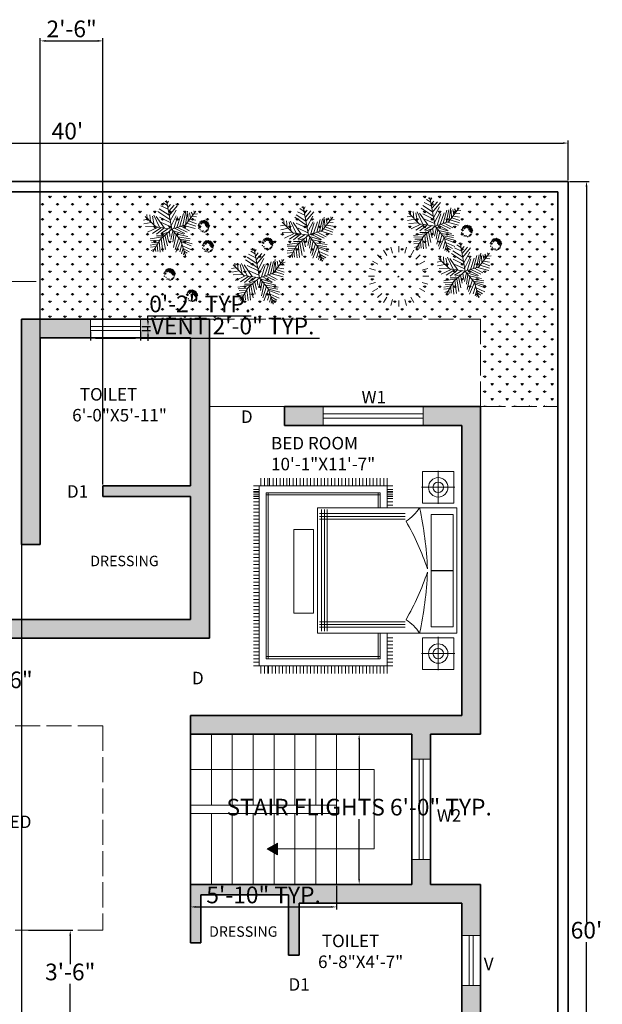
# Model space of a CAD drawing. Units: inches. Extents: x 1070 to 2371, y 645 to 1546.
# Tile 7 of 10: x 1379 to 1658, y 1014 to 1486. Entities that reach past the tile are written whole.
import ezdxf

# ---------------------------------------------------------------- set-up
doc = ezdxf.new("R2010")
doc.units = ezdxf.units.IN
doc.linetypes.add('ACAD_ISO02W100', pattern=[15, 12, -3])
for name, color, linetype, lineweight in [('A-ANNO-DIMS', 2, 'Continuous', 18), ('A-ANNO-SYMB', 7, 'Continuous', 18), ('A-ANNO-TEXT', 7, 'Continuous', 18), ('A-AREA-IDEN', 7, 'Continuous', 18), ('A-DOOR', 4, 'Continuous', 18), ('A-FLOR-OVHD', 8, 'ACAD_ISO02W100', 13), ('A-FLOR-STRS', 7, 'Continuous', 18), ('A-FURN', 8, 'Continuous', 18), ('A-GLAZ', 4, 'Continuous', 18), ('A-ROOF-OVHD', 8, 'ACAD_ISO02W100', 13), ('A-WALL', 7, 'Continuous', 35), ('C-PROP', 7, 'Continuous', 35), ('L-PLNT-BEDS-HIDN', 3, 'ACAD_ISO02W100', 13), ('L-PLNT-TREE', 94, 'Continuous', 13)]:
    doc.layers.add(name, color=color, linetype=linetype, lineweight=lineweight)
doc.layers.add('A-WALL-PATT', color=162, linetype='Continuous', lineweight=13, true_color=0x044ac3)
doc.layers.add('L-PLNT-PATT', color=85, linetype='Continuous', lineweight=13, true_color=0x58ba48)
doc.styles.get("Standard").update_dxf_attribs({"font": 'arial.ttf'})
doc.dimstyles.new('ISO-25', dxfattribs={"dimtxt": 8, "dimasz": 2.5, "dimexe": 1.25, "dimexo": 0.625, "dimtad": 1, "dimtih": 1, "dimtoh": 1, "dimdec": 1, "dimlunit": 3, "dimtxsty": 'Standard', "dimcen": 2.5, "dimadec": 0, "dimazin": 0, "dimtfac": 1, "dimtdec": 1, "dimtmove": 0, "dimatfit": 3, "dimfxl": 1, "dimarcsym": 0})

# ---------------------------------------------------------------- blocks, each defined once
blk = doc.blocks.new('A$C462B680F')
for p, q in [((0.011, 2.874, -0.291), (0.465, 2.874, -0.291)), ((0.011, 2.424, -0.291), (0.011, 2.874, -0.291)), ((0.238, 2.649, -0.561), (0.238, 2.887, -0.561)), ((0.465, 2.874, -0.291), (0.465, 2.424, -0.291)), ((2.33, 2.918, -0.291), (0.53, 2.918, -0.291)), ((0.53, 2.918, -0.291), (0.53, 0.918, -0.291)), ((1.434, 2.861, -0.291), (0.627, 2.861, -0.291)), ((0.627, 2.861, -0.291), (0.627, 2.55, -0.291)), ((1.43, 2.861, -0.291), (1.43, 2.55, -0.291)), ((2.237, 2.861, -0.291), (1.43, 2.861, -0.291)), ((1.434, 2.55, -0.291), (1.434, 2.861, -0.291)), ((2.237, 2.55, -0.291), (2.237, 2.861, -0.291)), ((2.33, 0.918, -0.291), (2.33, 2.918, -0.291)), ((2.849, 2.874, -0.291), (2.395, 2.874, -0.291)), ((2.395, 2.874, -0.291), (2.395, 2.424, -0.291)), ((2.622, 2.649, -0.561), (2.622, 2.887, -0.561)), ((2.849, 2.424, -0.291), (2.849, 2.874, -0.291)), ((0.238, 2.649, -0.561), (0, 2.649, -0.561)), ((0.238, 2.649, -0.561), (0.238, 2.411, -0.561)), ((0.238, 2.649, -0.561), (0.476, 2.649, -0.561)), ((0.627, 2.55, -0.291), (1.434, 2.55, -0.291)), ((1.43, 2.55, -0.291), (2.237, 2.55, -0.291)), ((2.622, 2.649, -0.561), (2.384, 2.649, -0.561)), ((2.622, 2.649, -0.561), (2.622, 2.411, -0.561)), ((2.622, 2.649, -0.561), (2.861, 2.649, -0.561)), ((0.465, 2.424, -0.291), (0.011, 2.424, -0.291)), ((2.395, 2.424, -0.291), (2.849, 2.424, -0.291)), ((0.615, 2.176, -0.291), (0.615, 0.947, -0.291)), ((0.655, 2.176, -0.291), (0.655, 0.947, -0.291)), ((0.695, 2.176, -0.291), (0.695, 0.947, -0.291)), ((2.165, 2.176, -0.291), (2.165, 0.947, -0.291)), ((2.205, 2.176, -0.291), (2.205, 0.947, -0.291)), ((2.245, 2.176, -0.291), (2.245, 0.947, -0.291)), ((0.219, 1.918, -0.291), (0.219, 2, -0.291)), ((0.269, 1.918, -0.291), (0.269, 2, -0.291)), ((0.296, 1.918, -0.291), (0.296, 2, -0.291)), ((0.319, 1.918, -0.291), (0.319, 2, -0.291)), ((0.346, 1.918, -0.291), (0.346, 2, -0.291)), ((0.369, 1.918, -0.291), (0.369, 2, -0.291)), ((0.396, 1.918, -0.291), (0.396, 2, -0.291)), ((0.446, 1.918, -0.291), (0.446, 2, -0.291)), ((0.496, 1.918, -0.291), (0.496, 2, -0.291)), ((2.396, 1.918, -0.291), (2.396, 2, -0.291)), ((2.446, 1.918, -0.291), (2.446, 2, -0.291)), ((2.496, 1.918, -0.291), (2.496, 2, -0.291)), ((2.546, 1.918, -0.291), (2.546, 2, -0.291)), ((2.596, 1.918, -0.291), (2.596, 2, -0.291)), ((2.646, 1.918, -0.291), (2.646, 2, -0.291)), ((2.696, 1.918, -0.291), (2.696, 2, -0.291)), ((2.746, 1.918, -0.291), (2.746, 2, -0.291)), ((2.796, 1.918, -0.291), (2.796, 2, -0.291)), ((0.215, 1.918, -0.291), (0.105, 1.918, -0.291)), ((0.215, 1.868, -0.291), (0.105, 1.868, -0.291)), ((0.215, 1.918, -0.291), (0.215, 0.082, -0.291)), ((0.53, 1.918, -0.291), (0.215, 1.918, -0.291)), ((2.33, 1.918, -0.291), (2.796, 1.918, -0.291)), ((2.796, 1.918, -0.291), (2.796, 0.082, -0.291)), ((2.796, 1.918, -0.291), (2.906, 1.918, -0.291)), ((2.796, 1.868, -0.291), (2.906, 1.868, -0.291)), ((0.215, 1.818, -0.291), (0.105, 1.818, -0.291)), ((0.215, 1.768, -0.291), (0.105, 1.768, -0.291)), ((0.215, 1.718, -0.291), (0.105, 1.718, -0.291)), ((0.315, 1.818, -0.291), (0.315, 0.182, -0.291)), ((0.53, 1.818, -0.291), (0.315, 1.818, -0.291)), ((0.53, 1.788, -0.291), (0.315, 1.788, -0.291)), ((0.345, 1.818, -0.291), (0.345, 0.182, -0.291)), ((2.33, 1.818, -0.291), (2.696, 1.818, -0.291)), ((2.33, 1.788, -0.291), (2.696, 1.788, -0.291)), ((2.666, 1.818, -0.291), (2.666, 0.182, -0.291)), ((2.696, 1.818, -0.291), (2.696, 0.182, -0.291)), ((2.796, 1.818, -0.291), (2.906, 1.818, -0.291)), ((2.796, 1.768, -0.291), (2.906, 1.768, -0.291)), ((2.796, 1.718, -0.291), (2.906, 1.718, -0.291)), ((0.215, 1.668, -0.291), (0.105, 1.668, -0.291)), ((0.215, 1.618, -0.291), (0.105, 1.618, -0.291)), ((0.215, 1.568, -0.291), (0.105, 1.568, -0.291)), ((2.796, 1.668, -0.291), (2.906, 1.668, -0.291)), ((2.796, 1.618, -0.291), (2.906, 1.618, -0.291)), ((2.796, 1.568, -0.291), (2.906, 1.568, -0.291)), ((0.215, 1.518, -0.291), (0.105, 1.518, -0.291)), ((0.215, 1.468, -0.291), (0.105, 1.468, -0.291)), ((0.215, 1.418, -0.291), (0.105, 1.418, -0.291)), ((2.796, 1.518, -0.291), (2.906, 1.518, -0.291)), ((2.796, 1.468, -0.291), (2.906, 1.468, -0.291)), ((2.796, 1.418, -0.291), (2.906, 1.418, -0.291)), ((0.215, 1.368, -0.291), (0.105, 1.368, -0.291)), ((0.215, 1.318, -0.291), (0.105, 1.318, -0.291)), ((2.796, 1.368, -0.291), (2.906, 1.368, -0.291)), ((2.796, 1.318, -0.291), (2.906, 1.318, -0.291)), ((0.215, 1.268, -0.291), (0.105, 1.268, -0.291)), ((0.215, 1.218, -0.291), (0.105, 1.218, -0.291)), ((0.215, 1.168, -0.291), (0.105, 1.168, -0.291)), ((2.796, 1.268, -0.291), (2.906, 1.268, -0.291)), ((2.796, 1.218, -0.291), (2.906, 1.218, -0.291)), ((2.796, 1.168, -0.291), (2.906, 1.168, -0.291)), ((0.215, 1.118, -0.291), (0.105, 1.118, -0.291)), ((0.215, 1.068, -0.291), (0.105, 1.068, -0.291)), ((0.215, 1.018, -0.291), (0.105, 1.018, -0.291)), ((0.558, 1.057, -0.291), (2.299, 1.057, -0.291)), ((0.558, 1.017, -0.291), (2.299, 1.017, -0.291)), ((2.796, 1.118, -0.291), (2.906, 1.118, -0.291)), ((2.796, 1.068, -0.291), (2.906, 1.068, -0.291)), ((2.796, 1.018, -0.291), (2.906, 1.018, -0.291)), ((0.215, 0.968, -0.291), (0.105, 0.968, -0.291)), ((0.215, 0.918, -0.291), (0.105, 0.918, -0.291)), ((0.215, 0.868, -0.291), (0.105, 0.868, -0.291)), ((0.53, 0.918, -0.291), (2.33, 0.918, -0.291)), ((0.558, 0.977, -0.291), (2.299, 0.977, -0.291)), ((0.844, 0.859, -0.291), (0.844, 0.579, -0.291)), ((2.044, 0.859, -0.291), (0.844, 0.859, -0.291)), ((2.044, 0.579, -0.291), (2.044, 0.859, -0.291)), ((2.796, 0.968, -0.291), (2.906, 0.968, -0.291)), ((2.796, 0.918, -0.291), (2.906, 0.918, -0.291)), ((2.796, 0.868, -0.291), (2.906, 0.868, -0.291)), ((0.215, 0.818, -0.291), (0.105, 0.818, -0.291)), ((0.215, 0.768, -0.291), (0.105, 0.768, -0.291)), ((0.215, 0.718, -0.291), (0.105, 0.718, -0.291)), ((2.796, 0.818, -0.291), (2.906, 0.818, -0.291)), ((2.796, 0.768, -0.291), (2.906, 0.768, -0.291)), ((2.796, 0.718, -0.291), (2.906, 0.718, -0.291)), ((0.215, 0.668, -0.291), (0.105, 0.668, -0.291)), ((0.215, 0.618, -0.291), (0.105, 0.618, -0.291)), ((0.215, 0.568, -0.291), (0.105, 0.568, -0.291)), ((0.844, 0.579, -0.291), (2.044, 0.579, -0.291)), ((2.796, 0.668, -0.291), (2.906, 0.668, -0.291)), ((2.796, 0.618, -0.291), (2.906, 0.618, -0.291)), ((2.796, 0.568, -0.291), (2.906, 0.568, -0.291)), ((0.215, 0.518, -0.291), (0.105, 0.518, -0.291)), ((0.215, 0.48, -0.291), (0.105, 0.48, -0.291)), ((0.215, 0.43, -0.291), (0.105, 0.43, -0.291)), ((2.796, 0.518, -0.291), (2.906, 0.518, -0.291)), ((2.796, 0.516, -0.291), (2.906, 0.516, -0.291)), ((2.796, 0.466, -0.291), (2.906, 0.466, -0.291)), ((0.215, 0.38, -0.291), (0.105, 0.38, -0.291)), ((0.215, 0.33, -0.291), (0.105, 0.33, -0.291)), ((2.796, 0.416, -0.291), (2.906, 0.416, -0.291)), ((2.796, 0.366, -0.291), (2.906, 0.366, -0.291)), ((2.796, 0.316, -0.291), (2.906, 0.316, -0.291)), ((0.215, 0.28, -0.291), (0.105, 0.28, -0.291)), ((0.215, 0.23, -0.291), (0.105, 0.23, -0.291)), ((0.215, 0.207, -0.291), (0.105, 0.207, -0.291)), ((0.215, 0.207, -0.291), (0.105, 0.207, -0.291)), ((0.215, 0.157, -0.291), (0.105, 0.157, -0.291)), ((2.696, 0.212, -0.291), (0.315, 0.212, -0.291)), ((2.696, 0.182, -0.291), (0.315, 0.182, -0.291)), ((2.796, 0.266, -0.291), (2.906, 0.266, -0.291)), ((2.796, 0.216, -0.291), (2.906, 0.216, -0.291)), ((2.796, 0.207, -0.291), (2.906, 0.207, -0.291)), ((2.796, 0.207, -0.291), (2.906, 0.207, -0.291)), ((2.796, 0.157, -0.291), (2.906, 0.157, -0.291)), ((0.215, 0.107, -0.291), (0.105, 0.107, -0.291)), ((2.796, 0.082, -0.291), (0.215, 0.082, -0.291)), ((0.219, 0.082, -0.291), (0.219, 0, -0.291)), ((0.269, 0.082, -0.291), (0.269, 0, -0.291)), ((0.296, 0.082, -0.291), (0.296, 0, -0.291)), ((0.319, 0.082, -0.291), (0.319, 0, -0.291)), ((0.346, 0.082, -0.291), (0.346, 0, -0.291)), ((0.369, 0.082, -0.291), (0.369, 0, -0.291)), ((0.396, 0.082, -0.291), (0.396, 0, -0.291)), ((0.446, 0.082, -0.291), (0.446, 0, -0.291)), ((0.496, 0.082, -0.291), (0.496, 0, -0.291)), ((0.546, 0.082, -0.291), (0.546, 0, -0.291)), ((0.596, 0.082, -0.291), (0.596, 0, -0.291)), ((0.646, 0.082, -0.291), (0.646, 0, -0.291)), ((0.696, 0.082, -0.291), (0.696, 0, -0.291)), ((0.746, 0.082, -0.291), (0.746, 0, -0.291)), ((0.796, 0.082, -0.291), (0.796, 0, -0.291)), ((0.846, 0.082, -0.291), (0.846, 0, -0.291)), ((0.896, 0.082, -0.291), (0.896, 0, -0.291)), ((0.946, 0.082, -0.291), (0.946, 0, -0.291)), ((0.996, 0.082, -0.291), (0.996, 0, -0.291)), ((1.046, 0.082, -0.291), (1.046, 0, -0.291)), ((1.096, 0.082, -0.291), (1.096, 0, -0.291)), ((1.146, 0.082, -0.291), (1.146, 0, -0.291)), ((1.196, 0.082, -0.291), (1.196, 0, -0.291)), ((1.246, 0.082, -0.291), (1.246, 0, -0.291)), ((1.296, 0.082, -0.291), (1.296, 0, -0.291)), ((1.346, 0.082, -0.291), (1.346, 0, -0.291)), ((1.346, 0.082, -0.291), (1.346, 0, -0.291)), ((1.396, 0.082, -0.291), (1.396, 0, -0.291)), ((1.396, 0.082, -0.291), (1.396, 0, -0.291)), ((1.446, 0.082, -0.291), (1.446, 0, -0.291)), ((1.446, 0.082, -0.291), (1.446, 0, -0.291)), ((1.496, 0.082, -0.291), (1.496, 0, -0.291)), ((1.496, 0.082, -0.291), (1.496, 0, -0.291)), ((1.546, 0.082, -0.291), (1.546, 0, -0.291)), ((1.596, 0.082, -0.291), (1.596, 0, -0.291)), ((1.646, 0.082, -0.291), (1.646, 0, -0.291)), ((1.696, 0.082, -0.291), (1.696, 0, -0.291)), ((1.746, 0.082, -0.291), (1.746, 0, -0.291)), ((1.796, 0.082, -0.291), (1.796, 0, -0.291)), ((1.846, 0.082, -0.291), (1.846, 0, -0.291)), ((1.846, 0.082, -0.291), (1.846, 0, -0.291)), ((1.896, 0.082, -0.291), (1.896, 0, -0.291)), ((1.946, 0.082, -0.291), (1.946, 0, -0.291)), ((1.996, 0.082, -0.291), (1.996, 0, -0.291)), ((2.046, 0.082, -0.291), (2.046, 0, -0.291)), ((2.096, 0.082, -0.291), (2.096, 0, -0.291)), ((2.146, 0.082, -0.291), (2.146, 0, -0.291)), ((2.196, 0.082, -0.291), (2.196, 0, -0.291)), ((2.246, 0.082, -0.291), (2.246, 0, -0.291)), ((2.296, 0.082, -0.291), (2.296, 0, -0.291)), ((2.346, 0.082, -0.291), (2.346, 0, -0.291)), ((2.396, 0.082, -0.291), (2.396, 0, -0.291)), ((2.446, 0.082, -0.291), (2.446, 0, -0.291)), ((2.496, 0.082, -0.291), (2.496, 0, -0.291)), ((2.546, 0.082, -0.291), (2.546, 0, -0.291)), ((2.596, 0.082, -0.291), (2.596, 0, -0.291)), ((2.646, 0.082, -0.291), (2.646, 0, -0.291)), ((2.696, 0.082, -0.291), (2.696, 0, -0.291)), ((2.746, 0.082, -0.291), (2.746, 0, -0.291)), ((2.796, 0.107, -0.291), (2.906, 0.107, -0.291)), ((2.796, 0.082, -0.291), (2.796, 0, -0.291))]:
    blk.add_line(p, q)
for centre, radius in [((0.238, 2.649, -0.561), 0.139), ((0.238, 2.649, -0.561), 0.075), ((2.622, 2.649, -0.561), 0.139), ((2.622, 2.649, -0.561), 0.075)]:
    blk.add_circle(centre, radius)
for centre, radius, start, end in [((1.618, -2.572, -0.291), 5.071, 92.3872, 102.3913), ((2.601, -1.074, -0.291), 3.763, 108.5127, 119.9306), ((1.243, -2.572, -0.291), 5.071, 77.6087, 87.6128), ((0.259, -1.074, -0.291), 3.763, 60.0694, 71.4873), ((0.231, 1.886, -0.291), 0.578, 31.4118, 58.8491), ((2.63, 1.886, -0.291), 0.578, 121.1509, 148.5882)]:
    blk.add_arc(centre, radius, start, end)
blk = doc.blocks.new('*U5')
for p, q in [((-5.114, 28.097), (-24.676, 40.636)), ((-7.288, 39.707), (-21.778, 46.673)), ((-8.737, 47.138), (-17.069, 52.711)), ((-10.186, 53.64), (-13.084, 55.962)), ((0, 0), (-10.5, 57)), ((-9.099, 51.782), (-6.563, 55.962)), ((-7.65, 43.423), (-2.578, 49.46)), ((-5.839, 35.992), (4.667, 48.067)), ((-5.114, 27.632), (10.463, 46.673)), ((-47.498, 19.737), (-55.83, 18.344)), ((-31.5, 4.5), (-52.5, 25.5)), ((-48.585, 21.131), (-49.309, 29.026)), ((-43.513, 28.561), (-42.427, 15.558)), ((-38.442, 26.239), (-34.819, 7.663)), ((-35.544, 28.097), (-24.314, 3.947)), ((-14.533, 2.09), (-30.834, 25.31)), ((-3.665, 19.273), (-27.574, 35.527)), ((-24.314, 23.917), (-2.941, 13.7)), ((-2.941, 16.486), (8.652, 37.85)), ((-1.129, 6.734), (9.014, 26.704)), ((3.942, 1.625), (11.187, 24.381)), ((10.101, 3.483), (17.708, 26.239)), ((16.259, 5.805), (23.142, 31.348)), ((22.055, 7.198), (27.489, 32.277)), ((27, 9), (48, 36)), ((27.127, 9.056), (31.112, 35.992)), ((31.836, 30.883), (32.561, 16.486)), ((35.096, 32.741), (37.27, 22.524)), ((36.183, 19.737), (48.137, 17.88)), ((38.719, 34.134), (41.979, 28.561)), ((40.53, 25.775), (48.862, 24.846)), ((43.791, 29.954), (51.036, 30.883)), ((44.153, 36.456), (45.239, 32.741)), ((-40.615, 13.7), (-55.105, 10.913)), ((-33.37, 6.269), (-52.207, 5.34)), ((-28.299, 3.483), (-47.86, -5.805)), ((-21.416, 3.018), (-38.079, -8.128)), ((0, 0), (-31.5, 4.5)), ((-15.982, 2.09), (-30.11, -9.521)), ((0, 0), (-22.5, -19.5)), ((-6.563, 1.161), (-21.416, -8.128)), ((-20.691, 13.7), (-1.129, 4.876)), ((0, 0), (27, 9)), ((0, 0), (18, -22.5)), ((6.478, 1.625), (26.04, -8.592)), ((11.187, 3.483), (30.749, -5.805)), ((18.07, 5.805), (35.096, -3.483)), ((24.229, 7.663), (46.688, 1.625)), ((29.662, 12.307), (48.137, 6.269)), ((33.285, 16.486), (48.862, 10.913)), ((-17.431, -15.094), (-42.789, -18.809)), ((-22.5, -19.5), (-37.5, -45)), ((-15.257, -12.772), (-30.11, -12.772)), ((-20.691, -18.345), (-17.793, -44.352)), ((-6.563, -5.805), (-19.967, -9.985)), ((-17.069, -15.094), (-12.721, -40.172)), ((-13.446, -11.378), (-8.737, -32.741)), ((-9.461, -8.592), (-6.201, -23.453)), ((-4.752, -3.483), (-3.665, -14.629)), ((2.493, -3.019), (-1.491, -20.202)), ((1.769, -2.555), (24.229, -9.521)), ((5.029, -6.27), (2.131, -25.775)), ((9.014, -11.378), (3.58, -35.992)), ((14.085, -16.951), (6.478, -40.172)), ((7.565, -9.056), (32.198, -14.629)), ((12.274, -15.094), (36.907, -18.809)), ((-28.299, -29.026), (-42.789, -31.348)), ((-24.314, -21.596), (-42.427, -22.06)), ((-30.834, -34.135), (-42.427, -35.528)), ((-26.849, -26.24), (-40.253, -25.775)), ((-32.646, -36.921), (-31.921, -44.352)), ((-29.023, -30.884), (-27.936, -43.887)), ((-25.038, -23.918), (-22.865, -45.281)), ((18.07, -22.524), (8.289, -45.745)), ((20.244, -30.419), (15.897, -44.816)), ((16.259, -19.738), (36.183, -22.989)), ((18, -22.5), (27, -52.5)), ((18.433, -22.524), (40.53, -29.026)), ((19.157, -25.311), (38.719, -33.206)), ((22.78, -37.85), (19.519, -48.532)), ((21.331, -32.741), (39.081, -40.636)), ((22.78, -38.314), (34.372, -44.816)), ((-34.457, -39.708), (-40.978, -42.494)), ((24.591, -45.745), (23.142, -50.854)), ((24.591, -43.423), (30.749, -47.603)), ((26.764, -49.925), (28.213, -50.854))]:
    blk.add_line(p, q)
blk = doc.blocks.new('*U6')
for p, q in [((-1.077, 60.601), (-1.077, 48.601)), ((-34.93, 34.454), (-43.503, 43.028)), ((-25.024, 42.079), (-31.077, 52.563)), ((-13.435, 46.72), (-16.606, 58.557)), ((11.28, 46.72), (14.452, 58.557)), ((22.87, 42.079), (28.923, 52.563)), ((32.776, 34.454), (41.349, 43.028)), ((-42.564, 24.554), (-53.039, 30.601)), ((40.409, 24.554), (50.884, 30.601)), ((-61.077, 0.601), (-49.077, 0.601)), ((-47.5, 13.04), (-59.033, 16.131)), ((45.346, 13.04), (56.878, 16.131)), ((58.923, 0.601), (46.923, 0.601)), ((-47.5, -11.837), (-59.033, -14.928)), ((45.346, -11.837), (56.878, -14.928)), ((-42.564, -23.351), (-53.039, -29.399)), ((-34.93, -33.251), (-43.503, -41.825)), ((32.776, -33.251), (41.349, -41.825)), ((40.409, -23.351), (50.884, -29.399)), ((-25.024, -40.876), (-31.077, -51.36)), ((-13.435, -45.517), (-16.606, -57.354)), ((-1.077, -59.399), (-1.077, -47.399)), ((11.28, -45.517), (14.452, -57.354)), ((22.87, -40.876), (28.923, -51.36))]:
    blk.add_line(p, q)
blk.add_lwpolyline([(-1.908, 0.978), (-2.67, -0.978), (0, 0)], close=True)
blk = doc.blocks.new('*U7')
for points in [[(-11.3, 1.8), (-9.8, 2.3), (-9.6, 3.4), (-10.4, 3.5)], [(-8.2, 0.4), (-9.4, 0.3), (-9.8, 0.8)], [(-8.1, 6), (-9.4, 5.9), (-9, 4.7)], [(-8.2, 3.1), (-8.5, 2.3), (-7.9, 2.6)], [(-5.8, 9.8), (-7.5, 9.2), (-8, 7.5), (-6.3, 8.5)], [(-7, 1.8), (-7.9, 1.5), (-7.5, 0.5)], [(-5.8, 6.8), (-6.7, 6.2), (-6.5, 5.7)], [(-4.6, 6.4), (-5.4, 4.5), (-3.9, 4.8)], [(-4.4, 11.1), (-5.2, 10.4), (-4, 9.5), (-2.1, 10.4)], [(-4.8, 8.6), (-3.8, 7.8), (-4, 9)], [(-2.9, 7.5), (-3.2, 6.6), (-2.3, 6.7)], [(-1.9, 9.5), (-2.5, 9), (-2.3, 8.5), (-1.8, 9.1)], [(-2, 11.7), (-1.6, 10.6), (-0.5, 10.1), (-0.2, 10.6), (-0.8, 11)], [(0, 9.1), (-1.3, 8.5), (-1.7, 7.2), (0.3, 7.8)], [(0.8, 7.2), (0.1, 6.5), (1.1, 5.9)], [(1.2, 12), (0.6, 11.3), (0.8, 10), (2.5, 11.1)], [(1.4, 8.5), (3.1, 8.8), (3.8, 7.8), (1.9, 7.8)], [(2.6, 9.9), (1.8, 9.8), (1.6, 9.2), (2.3, 9.4)], [(1.7, 6.3), (1.7, 7.1), (2.7, 7.5), (2.1, 6.9)], [(2.5, 6.8), (2.5, 5.9), (4.4, 5.2), (4.6, 6.7)], [(3.5, 1.9), (2.9, 3.5), (3.8, 3.5)], [(4.1, 11.1), (3.6, 10), (4, 9.2), (5.2, 8.7), (6.3, 9.4), (5.1, 10.2), (4.6, 10)], [(4.4, 4.6), (4.3, 3.7), (5.5, 3.3)], [(4.3, 2.7), (5.3, 2.7), (4.4, 1.3)], [(4.6, 8.3), (4.5, 7.8), (4.9, 7.6), (4.9, 8.3)], [(5.8, 1.5), (5, 0.4), (5.5, 0), (6.5, 0.4)], [(5.5, 5.5), (5.4, 4.8), (6.2, 5.1)], [(6.4, 7.9), (5.5, 7.7), (5.6, 6.2), (6.5, 6.6)], [(7.5, 1.7), (6.9, 1.3), (6.2, 2.1)], [(8.1, 5), (7.1, 4.6), (6.5, 4.1), (7.4, 3.1), (8.1, 3.5), (7.6, 3.9)], [(7.4, 9.3), (7.1, 7.9), (8.5, 7.9)], [(7.8, 6.8), (7.2, 6.2), (9, 5.5), (9.3, 6.4)], [(8.1, 0.8), (7.5, 0.1), (8.9, -0.3), (9.1, 0.5)], [(8.2, 2.6), (7.9, 2.1), (8.7, 1.5)], [(8.7, 4.7), (8.2, 4.6), (8.4, 3.9), (8.6, 4)], [(10.3, 5.2), (9.2, 4), (9, 2.3), (10.5, 0.5), (11.8, 0.4), (10.3, 2.5), (9.3, 2.4), (10.3, 2.8)], [(-10, -2.7), (-10.6, -3.3), (-10.4, -4.4), (-9.9, -3.5)], [(-8.3, -5.7), (-6.8, -5.3), (-7, -6.5)], [(-4.8, -8.8), (-4.4, -9.5), (-6, -9.8)], [(-2.5, -10.1), (-3, -10.2), (-1.8, -10.7)], [(-2.3, -9.2), (-1.3, -8.5), (-1, -9.5)], [(0.2, -10.6), (0.8, -11.3), (2.6, -11.4)], [(4.1, -9.5), (3.5, -10), (4.1, -10.6), (4.6, -9.9)], [(5.3, -8), (4.6, -8.2), (5, -8.9)], [(6, -9.5), (5.4, -10), (6.2, -10.1)], [(6.1, -8.9), (6.2, -7.2), (6.9, -6.7), (7.2, -7.4)], [(7.8, -0.8), (6.4, -1.5), (6.4, -0.7)], [(8.3, -1.8), (8, -2.5), (7.6, -2.1)], [(8.1, -8.1), (8.6, -7.1), (7.9, -7.6)], [(9.3, -5.1), (8.5, -6.3), (8, -5.2)], [(9.3, -1.8), (9.5, -3.7), (10.1, -2.5)], [(10.1, -0.6), (9.7, -1.3), (10.5, -0.9)]]:
    blk.add_lwpolyline(points, close=True)
blk = doc.blocks.new('*D11')
at = {"layer": 'A-ANNO-DIMS', "color": 0, "lineweight": -2, "transparency": 16777216}
for p, q in [((1162.11, 1409.4), (1162.11, 1428.36)), ((1164.61, 1427.11), (1639.61, 1427.11)), ((1642.11, 1409.4), (1642.11, 1428.36))]:
    blk.add_line(p, q, dxfattribs=at)
at = {"layer": 'A-ANNO-DIMS', "color": 0, "transparency": 16777216}
for points in [[(1164.61, 1427.53), (1164.61, 1426.7), (1162.11, 1427.11)], [(1639.61, 1427.53), (1639.61, 1426.7), (1642.11, 1427.11)]]:
    blk.add_solid(points, dxfattribs=at)
at = {"layer": 'Defpoints', "color": 0, "transparency": 16777216}
for p in [(1642.11, 1427.11), (1162.11, 1408.77), (1642.11, 1408.77)]:
    blk.add_point(p, dxfattribs=at)
at = {"layer": 'A-ANNO-DIMS', "color": 0, "transparency": 16777216, "insert": (1402.11, 1431.82), "char_height": 8, "attachment_point": 5}
blk.add_mtext("40'", dxfattribs=at)
blk = doc.blocks.new('*D12')
at = {"layer": 'A-ANNO-DIMS', "color": 0, "lineweight": -2, "transparency": 16777216}
for p, q in [((1642.74, 1408.77), (1652.12, 1408.77)), ((1650.87, 1406.27), (1650.87, 1053.48)), ((1650.87, 691.27), (1650.87, 1044.06)), ((1642.74, 688.77), (1652.12, 688.77))]:
    blk.add_line(p, q, dxfattribs=at)
at = {"layer": 'A-ANNO-DIMS', "color": 0, "transparency": 16777216}
for points in [[(1650.46, 1406.27), (1651.29, 1406.27), (1650.87, 1408.77)], [(1650.46, 691.27), (1651.29, 691.27), (1650.87, 688.77)]]:
    blk.add_solid(points, dxfattribs=at)
at = {"layer": 'Defpoints', "color": 0, "transparency": 16777216}
for p in [(1642.11, 1408.77), (1642.11, 688.77), (1650.87, 688.77)]:
    blk.add_point(p, dxfattribs=at)
at = {"layer": 'A-ANNO-DIMS', "color": 0, "transparency": 16777216, "insert": (1650.87, 1048.77), "char_height": 8, "attachment_point": 5}
blk.add_mtext("60'", dxfattribs=at)
blk = doc.blocks.new('*D13')
at = {"layer": 'A-ANNO-DIMS', "color": 0, "lineweight": -2, "transparency": 16777216}
for p, q in [((1366.14, 1189.77), (1374.63, 1189.77)), ((1373.38, 1187.27), (1373.38, 1173.48)), ((1373.38, 1150.27), (1373.38, 1164.06)), ((1366.14, 1147.77), (1374.63, 1147.77))]:
    blk.add_line(p, q, dxfattribs=at)
at = {"layer": 'A-ANNO-DIMS', "color": 0, "transparency": 16777216}
for points in [[(1372.97, 1187.27), (1373.8, 1187.27), (1373.38, 1189.77)], [(1372.97, 1150.27), (1373.8, 1150.27), (1373.38, 1147.77)]]:
    blk.add_solid(points, dxfattribs=at)
at = {"layer": 'Defpoints', "color": 0, "transparency": 16777216}
for p in [(1365.51, 1189.77), (1365.51, 1147.77), (1373.38, 1147.77)]:
    blk.add_point(p, dxfattribs=at)
at = {"layer": 'A-ANNO-DIMS', "color": 0, "transparency": 16777216, "insert": (1373.38, 1168.77), "char_height": 8, "attachment_point": 5}
blk.add_mtext('3\'-6"', dxfattribs=at)
blk = doc.blocks.new('*D14')
at = {"layer": 'A-ANNO-DIMS', "color": 0, "lineweight": -2, "transparency": 16777216}
for p, q in [((1383.51, 1049.77), (1404.69, 1049.77)), ((1403.44, 1047.27), (1403.44, 1033.48)), ((1403.44, 1010.27), (1403.44, 1024.06)), ((1395.74, 1007.77), (1404.69, 1007.77))]:
    blk.add_line(p, q, dxfattribs=at)
at = {"layer": 'A-ANNO-DIMS', "color": 0, "transparency": 16777216}
for points in [[(1403.02, 1047.27), (1403.86, 1047.27), (1403.44, 1049.77)], [(1403.02, 1010.27), (1403.86, 1010.27), (1403.44, 1007.77)]]:
    blk.add_solid(points, dxfattribs=at)
at = {"layer": 'Defpoints', "color": 0, "transparency": 16777216}
for p in [(1382.88, 1049.77), (1395.11, 1007.77), (1403.44, 1007.77)]:
    blk.add_point(p, dxfattribs=at)
at = {"layer": 'A-ANNO-DIMS', "color": 0, "transparency": 16777216, "insert": (1403.44, 1028.77), "char_height": 8, "attachment_point": 5}
blk.add_mtext('3\'-6"', dxfattribs=at)
blk = doc.blocks.new('GLAZ-48IN')
for p, q in [((0, 48), (0, 0)), ((2, 48), (2, 0))]:
    blk.add_line(p, q)
blk = doc.blocks.new('GLAZ-VENT-24IN')
for p, q in [((0, 2), (24, 2)), ((0, 0), (24, 0))]:
    blk.add_line(p, q)
blk = doc.blocks.new('STAIR-HALF-TURN')
for p, q in [((10, 72), (10, 38)), ((20, 72), (20, 38)), ((30, 72), (30, 38)), ((40, 72), (40, 38)), ((50, 72), (50, 38)), ((60, 72), (60, 38)), ((70, 72), (70, 0)), ((0, 38), (70, 38)), ((0, 34), (70, 34)), ((10, 34), (10, 0)), ((20, 34), (20, 0)), ((30, 34), (30, 0)), ((40, 34), (40, 18.86)), ((50, 34), (50, 0)), ((60, 34), (60, 0)), ((40, 15.14), (40, 0))]:
    blk.add_line(p, q)
blk = doc.blocks.new('STAIR-DIRECTION-RETURN')
h = blk.add_hatch(color=256)
h.dxf.hatch_style = 1
h.paths.add_polyline_path([(41.61, 5.58), (36.78, 2.79), (41.61, 0)])
for p, q in [((0, 40.79), (88.03, 40.79)), ((88.03, 40.79), (88.03, 2.79)), ((41.61, 2.79), (88.03, 2.79))]:
    blk.add_line(p, q)
blk.add_lwpolyline([(36.78, 2.79), (41.61, 0), (41.61, 5.58)], close=True)
blk = doc.blocks.new('*D29')
at = {"layer": 'A-ANNO-DIMS', "color": 0, "lineweight": -2, "transparency": 16777216}
for p, q in [((1413.11, 1336.65), (1413.11, 1332.42)), ((1437.11, 1336.65), (1437.11, 1332.42)), ((1415.61, 1333.67), (1434.61, 1333.67)), ((1437.11, 1333.67), (1522.95, 1333.67))]:
    blk.add_line(p, q, dxfattribs=at)
at = {"layer": 'A-ANNO-DIMS', "color": 0, "transparency": 16777216}
for points in [[(1415.61, 1334.09), (1415.61, 1333.26), (1413.11, 1333.67)], [(1434.61, 1334.09), (1434.61, 1333.26), (1437.11, 1333.67)]]:
    blk.add_solid(points, dxfattribs=at)
at = {"layer": 'Defpoints', "color": 0, "transparency": 16777216}
for p in [(1413.11, 1337.27), (1437.11, 1337.27), (1437.11, 1333.67)]:
    blk.add_point(p, dxfattribs=at)
at = {"layer": 'A-ANNO-DIMS', "color": 0, "transparency": 16777216, "insert": (1481.28, 1338.38), "char_height": 8, "attachment_point": 5}
blk.add_mtext('VENT 2\'-0" TYP.', dxfattribs=at)
blk = doc.blocks.new('*D30')
at = {"layer": 'A-ANNO-DIMS', "color": 0, "lineweight": -2, "transparency": 16777216}
for p, q in [((1440.71, 1341.77), (1440.71, 1344.27)), ((1440.71, 1344.27), (1490.1, 1344.27)), ((1437.74, 1339.27), (1441.96, 1339.27)), ((1437.74, 1337.27), (1441.96, 1337.27)), ((1440.71, 1337.27), (1440.71, 1339.27)), ((1440.71, 1334.77), (1440.71, 1332.27))]:
    blk.add_line(p, q, dxfattribs=at)
at = {"layer": 'A-ANNO-DIMS', "color": 0, "transparency": 16777216}
for points in [[(1440.3, 1341.77), (1441.13, 1341.77), (1440.71, 1339.27)], [(1440.3, 1334.77), (1441.13, 1334.77), (1440.71, 1337.27)]]:
    blk.add_solid(points, dxfattribs=at)
at = {"layer": 'Defpoints', "color": 0, "transparency": 16777216}
for p in [(1437.11, 1339.27), (1437.11, 1337.27), (1440.71, 1339.27)]:
    blk.add_point(p, dxfattribs=at)
at = {"layer": 'A-ANNO-DIMS', "color": 0, "transparency": 16777216, "insert": (1465.72, 1348.98), "char_height": 8, "attachment_point": 5}
blk.add_mtext('0\'-2" TYP.', dxfattribs=at)
blk = doc.blocks.new('*D43')
at = {"layer": 'A-ANNO-DIMS', "color": 0, "lineweight": -2, "transparency": 16777216}
for p, q in [((1531.74, 1143.77), (1543.16, 1143.77)), ((1541.91, 1141.27), (1541.91, 1112.53)), ((1541.91, 1074.27), (1541.91, 1103.01)), ((1531.74, 1071.77), (1543.16, 1071.77))]:
    blk.add_line(p, q, dxfattribs=at)
at = {"layer": 'A-ANNO-DIMS', "color": 0, "transparency": 16777216}
for points in [[(1541.5, 1141.27), (1542.33, 1141.27), (1541.91, 1143.77)], [(1541.5, 1074.27), (1542.33, 1074.27), (1541.91, 1071.77)]]:
    blk.add_solid(points, dxfattribs=at)
at = {"layer": 'Defpoints', "color": 0, "transparency": 16777216}
for p in [(1531.11, 1143.77), (1541.91, 1143.77), (1531.11, 1071.77)]:
    blk.add_point(p, dxfattribs=at)
at = {"layer": 'A-ANNO-DIMS', "color": 0, "transparency": 16777216, "insert": (1541.91, 1107.77), "char_height": 8, "attachment_point": 5}
blk.add_mtext('STAIR FLIGHTS 6\'-0" TYP.', dxfattribs=at)
blk = doc.blocks.new('*D44')
at = {"layer": 'A-ANNO-DIMS', "color": 0, "lineweight": -2, "transparency": 16777216}
for p, q in [((1461.11, 1071.15), (1461.11, 1059.72)), ((1531.11, 1071.15), (1531.11, 1059.72)), ((1463.61, 1060.97), (1528.61, 1060.97))]:
    blk.add_line(p, q, dxfattribs=at)
at = {"layer": 'A-ANNO-DIMS', "color": 0, "transparency": 16777216}
for points in [[(1463.61, 1061.39), (1463.61, 1060.56), (1461.11, 1060.97)], [(1528.61, 1061.39), (1528.61, 1060.56), (1531.11, 1060.97)]]:
    blk.add_solid(points, dxfattribs=at)
at = {"layer": 'Defpoints', "color": 0, "transparency": 16777216}
for p in [(1461.11, 1071.77), (1531.11, 1071.77), (1531.11, 1060.97)]:
    blk.add_point(p, dxfattribs=at)
at = {"layer": 'A-ANNO-DIMS', "color": 0, "transparency": 16777216, "insert": (1496.11, 1065.68), "char_height": 8, "attachment_point": 5}
blk.add_mtext('5\'-10" TYP.', dxfattribs=at)
blk = doc.blocks.new('*D49')
at = {"layer": 'A-ANNO-DIMS', "color": 0, "lineweight": -2, "transparency": 16777216}
for p, q in [((1344.11, 1342.15), (1344.11, 647.32)), ((1380.11, 1342.15), (1380.11, 647.32)), ((1346.61, 648.57), (1377.61, 648.57))]:
    blk.add_line(p, q, dxfattribs=at)
at = {"layer": 'A-ANNO-DIMS', "color": 0, "transparency": 16777216}
for points in [[(1346.61, 648.99), (1346.61, 648.16), (1344.11, 648.57)], [(1377.61, 648.99), (1377.61, 648.16), (1380.11, 648.57)]]:
    blk.add_solid(points, dxfattribs=at)
at = {"layer": 'Defpoints', "color": 0, "transparency": 16777216}
for p in [(1344.11, 1342.77), (1380.11, 1342.77), (1380.11, 648.57)]:
    blk.add_point(p, dxfattribs=at)
at = {"layer": 'A-ANNO-DIMS', "color": 0, "transparency": 16777216, "insert": (1362.11, 653.28), "char_height": 8, "attachment_point": 5}
blk.add_mtext('3\'-0"', dxfattribs=at)
blk = doc.blocks.new('*D50')
at = {"layer": 'A-ANNO-DIMS', "color": 0, "lineweight": -2, "transparency": 16777216}
for p, q in [((1389.11, 1235.4), (1389.11, 1477.34)), ((1419.11, 1263.4), (1419.11, 1477.34)), ((1391.61, 1476.09), (1416.61, 1476.09))]:
    blk.add_line(p, q, dxfattribs=at)
at = {"layer": 'A-ANNO-DIMS', "color": 0, "transparency": 16777216}
for points in [[(1391.61, 1476.51), (1391.61, 1475.68), (1389.11, 1476.09)], [(1416.61, 1476.51), (1416.61, 1475.68), (1419.11, 1476.09)]]:
    blk.add_solid(points, dxfattribs=at)
at = {"layer": 'Defpoints', "color": 0, "transparency": 16777216}
for p in [(1419.11, 1476.09), (1419.11, 1262.77), (1389.11, 1234.77)]:
    blk.add_point(p, dxfattribs=at)
at = {"layer": 'A-ANNO-DIMS', "color": 0, "transparency": 16777216, "insert": (1404.11, 1480.8), "char_height": 8, "attachment_point": 5}
blk.add_mtext('2\'-6"', dxfattribs=at)

msp = doc.modelspace()

# ---------------------------------------------------------------- hatches: boundary and pattern name
at = {"layer": 'A-WALL-PATT'}
h = msp.add_hatch(color=256, dxfattribs=at)
h.dxf.hatch_style = 1
h.paths.add_polyline_path([(1245.11, 1097.27), (1236.11, 1097.27), (1236.11, 1043.77), (1245.11, 1043.77)])
h.paths.add_polyline_path([(1245.11, 1198.77), (1207.11, 1198.77), (1207.11, 1333.77), (1245.61, 1333.77), (1245.61, 1342.77), (1198.11, 1342.77), (1198.11, 1189.77), (1236.11, 1189.77), (1236.11, 1145.27), (1245.11, 1145.27)])
h.paths.add_polyline_path([(1344.11, 1342.77), (1305.61, 1342.77), (1305.61, 1333.77), (1344.11, 1333.77)], flags=0)
h.paths.add_polyline_path([(1413.11, 1342.77), (1380.11, 1342.77), (1380.11, 1234.77), (1389.11, 1234.77), (1389.11, 1333.77), (1413.11, 1333.77)], flags=17)
h.paths.add_polyline_path([(1470.11, 1342.77), (1437.11, 1342.77), (1437.11, 1333.77), (1461.11, 1333.77), (1461.11, 1262.77), (1419.11, 1262.77), (1419.11, 1257.77), (1461.11, 1257.77), (1461.11, 1198.77), (1380.11, 1198.77), (1281.11, 1198.77), (1281.11, 1189.77), (1470.11, 1189.77)])
h.paths.add_polyline_path([(1524.61, 1300.77), (1506.11, 1300.77), (1506.11, 1291.77), (1524.61, 1291.77)], flags=17)
h.paths.add_polyline_path([(1600.11, 1300.77), (1572.61, 1300.77), (1572.61, 1291.77), (1591.11, 1291.77), (1591.11, 1152.77), (1461.11, 1152.77), (1461.11, 1143.77), (1567.11, 1143.77), (1567.11, 1131.77), (1576.11, 1131.77), (1576.11, 1143.77), (1600.11, 1143.77)])
h.paths.add_polyline_path([(1600.11, 1071.77), (1576.11, 1071.77), (1576.11, 1083.77), (1567.11, 1083.77), (1567.11, 1071.77), (1461.11, 1071.77), (1461.11, 1043.77), (1466.11, 1043.77), (1466.11, 1066.77), (1508.11, 1066.77), (1508.11, 1037.77), (1513.11, 1037.77), (1513.11, 1062.77), (1591.11, 1062.77), (1591.11, 1047.27), (1600.11, 1047.27)])
h.paths.add_polyline_path([(1600.11, 1023.27), (1591.11, 1023.27), (1591.11, 1007.77), (1461.11, 1007.77), (1461.11, 1002.77), (1591.11, 1002.77), (1591.11, 813.77), (1550.11, 813.77), (1550.11, 804.77), (1600.11, 804.77)])
h.paths.add_polyline_path([(1502.11, 813.77), (1461.11, 813.77), (1461.11, 804.77), (1502.11, 804.77)], flags=0)
h.paths.add_polyline_path([(1419.11, 1007.77), (1395.11, 1007.77), (1395.11, 998.77), (1410.11, 998.77), (1410.11, 916.77), (1395.11, 916.77), (1395.11, 907.77), (1410.11, 907.77), (1410.11, 804.77), (1419.11, 804.77)])
at = {"layer": 'L-PLNT-PATT'}
h = msp.add_hatch(dxfattribs=at)
h.set_pattern_fill('GRASS', color=256, scale=0.2)
h.paths.add_polyline_path([(1637.11, 1403.77), (1389.11, 1403.77), (1389.11, 1342.77), (1470.11, 1342.77), (1600.11, 1342.77), (1600.11, 1300.77), (1637.11, 1300.77)])

# ---------------------------------------------------------------- linework, layer by layer
at = {"layer": 'A-DOOR'}
msp.add_line((1506.11, 1300.77), (1470.11, 1300.77), dxfattribs=at)
at = {"layer": 'A-FLOR-OVHD'}
for p, q in [((1287.11, 1147.77), (1419.11, 1147.77)), ((1419.11, 1147.77), (1419.11, 1049.77)), ((1287.11, 1049.77), (1419.11, 1049.77))]:
    msp.add_line(p, q, dxfattribs=at)
at = {"layer": 'A-GLAZ'}
for p, q in [((1413.11, 1333.77), (1413.11, 1342.77)), ((1437.11, 1333.77), (1437.11, 1342.77)), ((1524.61, 1291.77), (1524.61, 1300.77)), ((1572.61, 1291.77), (1572.61, 1300.77)), ((1567.11, 1131.77), (1576.11, 1131.77)), ((1567.11, 1083.77), (1576.11, 1083.77)), ((1591.11, 1047.27), (1600.11, 1047.27)), ((1591.11, 1023.27), (1600.11, 1023.27))]:
    msp.add_line(p, q, dxfattribs=at)
at = {"layer": 'A-ROOF-OVHD'}
for p, q in [((1180.11, 1360.77), (1389.11, 1360.77)), ((1470.11, 1342.77), (1600.11, 1342.77)), ((1600.11, 1342.77), (1600.11, 1300.77))]:
    msp.add_line(p, q, dxfattribs=at)
at = {"layer": 'A-WALL'}
for p, q in [((1380.11, 1342.77), (1380.11, 1234.77)), ((1380.11, 1342.77), (1470.11, 1342.77)), ((1470.11, 1342.77), (1470.11, 1189.77)), ((1389.11, 1333.77), (1461.11, 1333.77)), ((1389.11, 1333.77), (1389.11, 1234.77)), ((1461.11, 1333.77), (1461.11, 1262.77)), ((1506.11, 1300.77), (1600.11, 1300.77)), ((1506.11, 1300.77), (1506.11, 1291.77)), ((1600.11, 1300.77), (1600.11, 1143.77)), ((1506.11, 1291.77), (1591.11, 1291.77)), ((1591.11, 1291.77), (1591.11, 1152.77)), ((1419.11, 1262.77), (1461.11, 1262.77)), ((1419.11, 1262.77), (1419.11, 1257.77)), ((1419.11, 1257.77), (1461.11, 1257.77)), ((1461.11, 1257.77), (1461.11, 1198.77)), ((1380.11, 1234.77), (1389.11, 1234.77)), ((1281.11, 1198.77), (1380.11, 1198.77)), ((1380.11, 1198.77), (1461.11, 1198.77)), ((1281.11, 1189.77), (1470.11, 1189.77)), ((1461.11, 1152.77), (1591.11, 1152.77)), ((1461.11, 1152.77), (1461.11, 1143.77)), ((1461.11, 1143.77), (1567.11, 1143.77)), ((1461.11, 1143.77), (1461.11, 1043.77)), ((1567.11, 1143.77), (1567.11, 1071.77)), ((1576.11, 1143.77), (1576.11, 1071.77)), ((1576.11, 1143.77), (1600.11, 1143.77)), ((1461.11, 1071.77), (1567.11, 1071.77)), ((1576.11, 1071.77), (1600.11, 1071.77)), ((1600.11, 1071.77), (1600.11, 804.77)), ((1466.11, 1066.77), (1466.11, 1043.77)), ((1466.11, 1066.77), (1508.11, 1066.77)), ((1508.11, 1066.77), (1508.11, 1037.77)), ((1513.11, 1062.77), (1513.11, 1037.77)), ((1513.11, 1062.77), (1591.11, 1062.77)), ((1591.11, 1062.77), (1591.11, 1007.77)), ((1461.11, 1043.77), (1466.11, 1043.77)), ((1508.11, 1037.77), (1513.11, 1037.77))]:
    msp.add_line(p, q, dxfattribs=at)
at = {"layer": 'C-PROP'}
for p, q in [((1162.11, 1408.77), (1642.11, 1408.77)), ((1642.11, 1408.77), (1642.11, 688.77)), ((1167.11, 1403.77), (1637.11, 1403.77)), ((1637.11, 1403.77), (1637.11, 693.77))]:
    msp.add_line(p, q, dxfattribs=at)
at = {"layer": 'L-PLNT-BEDS-HIDN'}
for p, q in [((1389.11, 1403.77), (1389.11, 1342.77)), ((1600.11, 1300.77), (1637.11, 1300.77))]:
    msp.add_line(p, q, dxfattribs=at)

# ---------------------------------------------------------------- block references
at = {"layer": 'A-ANNO-SYMB'}
msp.add_blockref('STAIR-DIRECTION-RETURN', (1461.11, 1085.98), dxfattribs=at)
at = {"layer": 'A-FLOR-STRS'}
msp.add_blockref('STAIR-HALF-TURN', (1461.11, 1071.77), dxfattribs=at)
at = {"layer": 'A-FURN', "xscale": 33.42019788357461, "yscale": 33.42019788357461, "zscale": 33.42019788357461, "rotation": 270}
msp.add_blockref('A$C462B680F', (1491.28, 1270.06, 9.72), dxfattribs=at)
at = {"layer": 'A-GLAZ'}
msp.add_blockref('GLAZ-VENT-24IN', (1413.11, 1337.27), dxfattribs=at)
for name, p, rotation in [('GLAZ-48IN', (1572.61, 1295.27), 90.00000000000003), ('GLAZ-48IN', (1572.61, 1131.77), 180), ('GLAZ-VENT-24IN', (1596.61, 1023.27), 90.00000000000328)]:
    msp.add_blockref(name, p, dxfattribs=dict(at, rotation=rotation))
at = {"layer": 'L-PLNT-TREE', "xscale": 0.2412959654679437, "yscale": 0.2412959654679437, "zscale": 0.2412959654679437}
for name, p in [('*U5', (1452.09, 1385.81)), ('*U5', (1578.33, 1387.35)), ('*U5', (1517.66, 1382.97)), ('*U7', (1467.42, 1387.19)), ('*U7', (1593.57, 1384.91)), ('*U7', (1469.46, 1377.56)), ('*U7', (1498.04, 1378.85)), ('*U5', (1592.79, 1365.68)), ('*U7', (1607.44, 1378.57)), ('*U5', (1494.17, 1362.59)), ('*U6', (1561.15, 1363.11)), ('*U7', (1451.04, 1364.17)), ('*U7', (1461.74, 1353.9))]:
    msp.add_blockref(name, p, dxfattribs=at)

# ---------------------------------------------------------------- texts
at = {"layer": 'A-ANNO-TEXT', "char_height": 6, "attachment_point": 1}
for s, insert in [('W1', (1543.06, 1308.32)), ('D', (1485.24, 1298.96)), ('D1', (1401.85, 1263.12)), ('D', (1461.78, 1173.67)), ('W2', (1579.12, 1107.82)), ('V', (1601.63, 1036.65)), ('D1', (1508.04, 1026.82))]:
    msp.add_mtext_dynamic_manual_height_columns(s, width=20.5094, gutter_width=12.5, heights=[0], dxfattribs=dict(at, insert=insert))
at = {"layer": 'A-AREA-IDEN', "attachment_point": 1}
for s, width, gutter_width, heights, insert, char_height in [('  TOILET\\P6\'-0"X5\'-11"', 40.1799, 12.5, [0], (1404.37, 1309.68), 6), ('BED ROOM\\P10\'-1"X11\'-7"', 101.5007, 0, [38.75], (1499.68, 1286.26), 6), ('DRESSING', 34.3208, 12.5, [0], (1413.03, 1229.31), 5), ('  DINING/LIVING\\PDOUBLE HIGHTED\\P   18\'-0"X16\'-6"', 97.1991, 12.5, [0], (1315.46, 1114.77), 6), ('DRESSING', 34.3208, 12.5, [0], (1469.98, 1051.66), 5), (' TOILET\\P6\'-8"X4\'-7"', 40.0374, 12.5, [0], (1522.2, 1047.69), 6)]:
    msp.add_mtext_dynamic_manual_height_columns(s, width=width, gutter_width=gutter_width, heights=heights, dxfattribs=dict(at, insert=insert, char_height=char_height))

# ---------------------------------------------------------------- dimensions: what is measured, and where the dimension line sits
at = {"layer": 'A-ANNO-DIMS'}
for base, p1, p2, override, picture, middle in [((1419.11, 1476.09), (1389.11, 1234.77), (1419.11, 1262.77), {"dimdec": 1, "dimlfac": 1, "dimrnd": 0, "dimzin": 1, "dimdsep": 46, "dimlunit": 4, "dimfrac": 2}, '*D50', (1404.11, 1480.8)), ((1642.11, 1427.11), (1162.11, 1408.77), (1642.11, 1408.77), {"dimclrd": 0, "dimclre": 0, "dimclrt": 0}, '*D11', (1402.11, 1431.82)), ((1380.11, 648.57), (1344.11, 1342.77), (1380.11, 1342.77), {"dimdec": 1, "dimlfac": 1, "dimrnd": 0, "dimzin": 1, "dimdsep": 46, "dimlunit": 4, "dimfrac": 2}, '*D49', (1362.11, 653.28))]:
    dim = msp.add_linear_dim(base=base, p1=p1, p2=p2, dimstyle='ISO-25', override=override, dxfattribs=at)
    dim.commit()
    dim.dimension.update_dxf_attribs({"geometry": picture, "text_midpoint": middle})
for base, p1, p2, picture, middle in [((1650.87, 688.77), (1642.11, 1408.77), (1642.11, 688.77), '*D12', (1650.87, 1048.77)), ((1373.38, 1147.77), (1365.51, 1189.77), (1365.51, 1147.77), '*D13', (1373.38, 1168.77)), ((1403.44, 1007.77), (1382.88, 1049.77), (1395.11, 1007.77), '*D14', (1403.44, 1028.77))]:
    dim = msp.add_linear_dim(base=base, p1=p1, p2=p2, angle=90, dimstyle='ISO-25', override={"dimclrd": 0, "dimclre": 0, "dimclrt": 0}, dxfattribs=at)
    dim.commit()
    dim.dimension.update_dxf_attribs({"geometry": picture, "text_midpoint": middle})
for base, p1, p2, text, picture, middle in [((1440.71, 1339.27), (1437.11, 1337.27), (1437.11, 1339.27), '<> TYP.', '*D30', (1465.72, 1348.98)), ((1541.91, 1143.77), (1531.11, 1071.77), (1531.11, 1143.77), 'STAIR FLIGHTS <> TYP.', '*D43', (1541.91, 1107.77))]:
    dim = msp.add_linear_dim(base=base, p1=p1, p2=p2, angle=90, text=text, dimstyle='ISO-25', override={"dimdec": 1, "dimlfac": 1, "dimrnd": 0, "dimzin": 1, "dimdsep": 46, "dimlunit": 4, "dimfrac": 2}, dxfattribs=at)
    dim.commit()
    dim.dimension.update_dxf_attribs({"geometry": picture, "text_midpoint": middle})
for base, p1, p2, text, picture, middle in [((1437.11, 1333.67), (1413.11, 1337.27), (1437.11, 1337.27), 'VENT <> TYP.', '*D29', (1481.28, 1338.38)), ((1531.11, 1060.97), (1461.11, 1071.77), (1531.11, 1071.77), '<> TYP.', '*D44', (1496.11, 1065.68))]:
    dim = msp.add_linear_dim(base=base, p1=p1, p2=p2, text=text, dimstyle='ISO-25', override={"dimdec": 1, "dimlfac": 1, "dimrnd": 0, "dimzin": 1, "dimdsep": 46, "dimlunit": 4, "dimfrac": 2}, dxfattribs=at)
    dim.commit()
    dim.dimension.update_dxf_attribs({"geometry": picture, "text_midpoint": middle})

doc.saveas('drawing.dxf')
